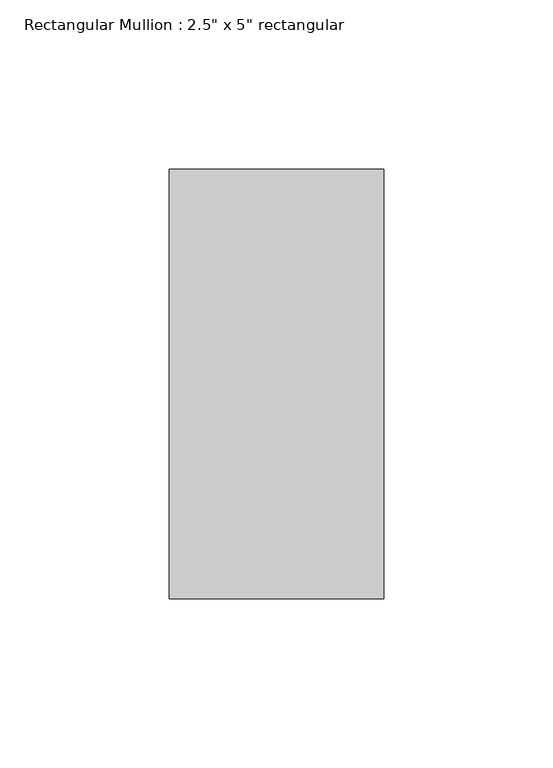
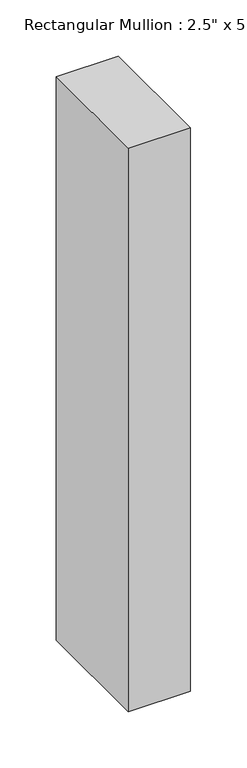
"""IFC4 building model written with IfcOpenShell, lengths in millimetres: member geometry."""

from ifc_helpers import new_model, si_unit, frame, origin, place, context, project, spatial, polyline, outline, extrude, source, transform, mapped, element, save


def member_6e77e263(model_context):
    return source(origin(), model_context, "Body", "SweptSolid", [
        extrude(outline(polyline([(31.75, 63.5), (31.75, -63.5), (-31.75, -63.5), (-31.75, 63.5), (31.75, 63.5)])), frame((0.0, 0.0, -609.6), z_axis=(0.0, 0.0, 1.0), x_axis=(1.0, 0.0, 0.0)), (0.0, 0.0, 1.0), 609.6),
    ])


if __name__ == "__main__":
    model = new_model("IFC4")
    model_context = context("Model", 3, world=origin())
    ifc_project = project(units=[si_unit("LENGTHUNIT", "METRE", prefix="MILLI")], contexts=[model_context])
    site = spatial("IfcSite", under=ifc_project)
    building = spatial("IfcBuilding", under=site)
    placement = place(None, origin())
    member_shape = member_6e77e263(model_context)
    element("IfcMember", 1, ObjectType="Rectangular Mullion : 2.5\" x 5\" rectangular", at=placement, inside=building, context=model_context, shape_type="MappedRepresentation", body=[
        mapped(member_shape, transform((0.0, 0.0, 0.0), x_axis=(1.0, 0.0, 0.0), y_axis=(0.0, 1.0, 0.0), z_axis=(0.0, 0.0, 1.0))),
    ])
    save(model, "model.ifc")

# Revit data of these elements
# Type "Rectangular Mullion : 2.5\" x 5\" rectangular"
#   built-in parameter 1007304 = 0.416667 (stored number, unit not read)
#   built-in parameter 1007301 = 0.104167 (stored number, unit not read)
#   built-in parameter 1007300 = 0.104167 (stored number, unit not read)
# Element 1 (IfcMember, "Rectangular Mullion : 2.5\" x 5\" rectangular")
#   Materials on its faces: "BLACK MATERIAL"
# Materials
#   "BLACK MATERIAL": class "Generic", colour RGB 120 120 120, transparency 0, Cost = 0
